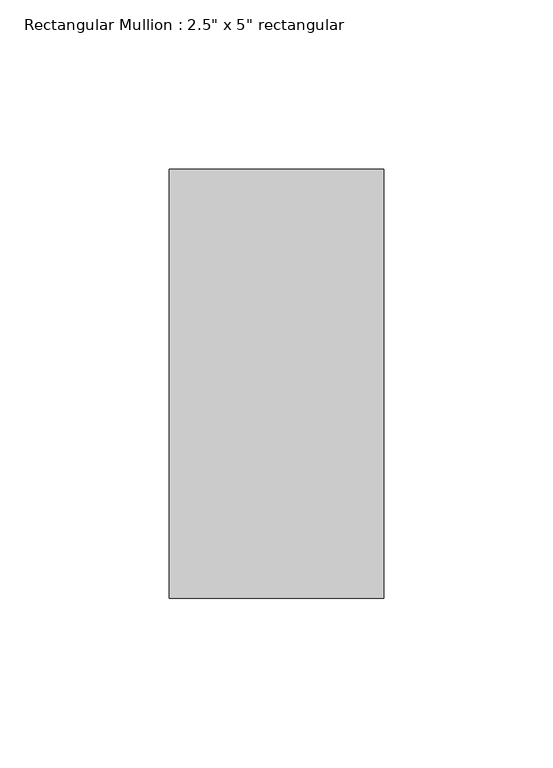
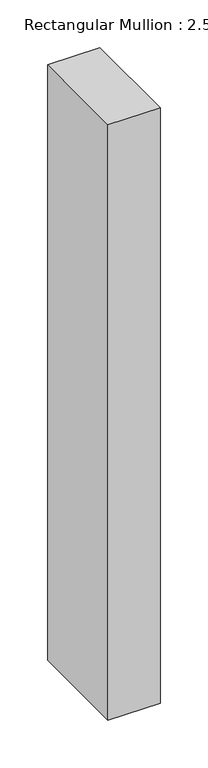
"""IFC4 building model written with IfcOpenShell, lengths in millimetres: member geometry."""

from ifc_helpers import new_model, si_unit, frame, origin, place, context, project, spatial, polyline, outline, extrude, source, transform, mapped, element, save


def member_2c21e81d(model_context):
    return source(origin(), model_context, "Body", "SweptSolid", [
        extrude(outline(polyline([(31.75, 63.5), (31.75, -63.5), (-31.75, -63.5), (-31.75, 63.5), (31.75, 63.5)])), frame((0.0, 0.0, -764.1166667), z_axis=(0.0, 0.0, 1.0), x_axis=(1.0, 0.0, 0.0)), (0.0, 0.0, 1.0), 764.1166667),
    ])


if __name__ == "__main__":
    model = new_model("IFC4")
    model_context = context("Model", 3, world=origin())
    ifc_project = project(units=[si_unit("LENGTHUNIT", "METRE", prefix="MILLI")], contexts=[model_context])
    site = spatial("IfcSite", under=ifc_project)
    building = spatial("IfcBuilding", under=site)
    placement = place(None, origin())
    member_shape = member_2c21e81d(model_context)
    element("IfcMember", 1, ObjectType="Rectangular Mullion : 2.5\" x 5\" rectangular", at=placement, inside=building, context=model_context, shape_type="MappedRepresentation", body=[
        mapped(member_shape, transform((0.0, 0.0, 0.0), x_axis=(1.0, 0.0, 0.0), y_axis=(0.0, 1.0, 0.0), z_axis=(0.0, 0.0, 1.0))),
    ])
    save(model, "model.ifc")

# Revit data of these elements
# Type "Rectangular Mullion : 2.5\" x 5\" rectangular"
#   built-in parameter 1007304 = 0.416667 (stored number, unit not read)
#   built-in parameter 1007301 = 0.104167 (stored number, unit not read)
#   built-in parameter 1007300 = 0.104167 (stored number, unit not read)
# Element 1 (IfcMember, "Rectangular Mullion : 2.5\" x 5\" rectangular")
#   Materials on its faces: "Aluminum"
# Materials
#   "Aluminum": class "Metal", colour RGB 247 247 247, transparency 0, Description = "Aluminum 6061", Cost = 0
